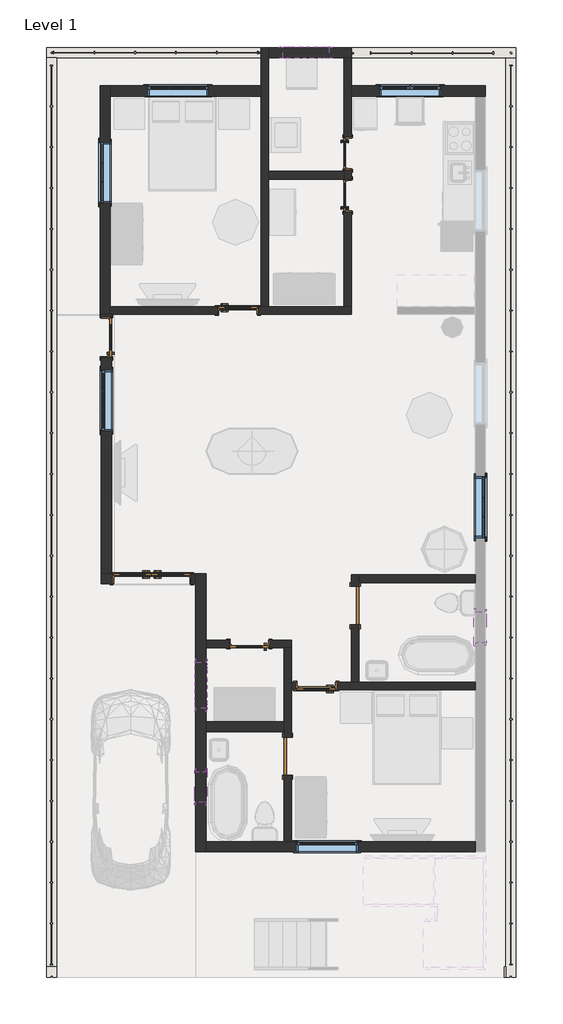
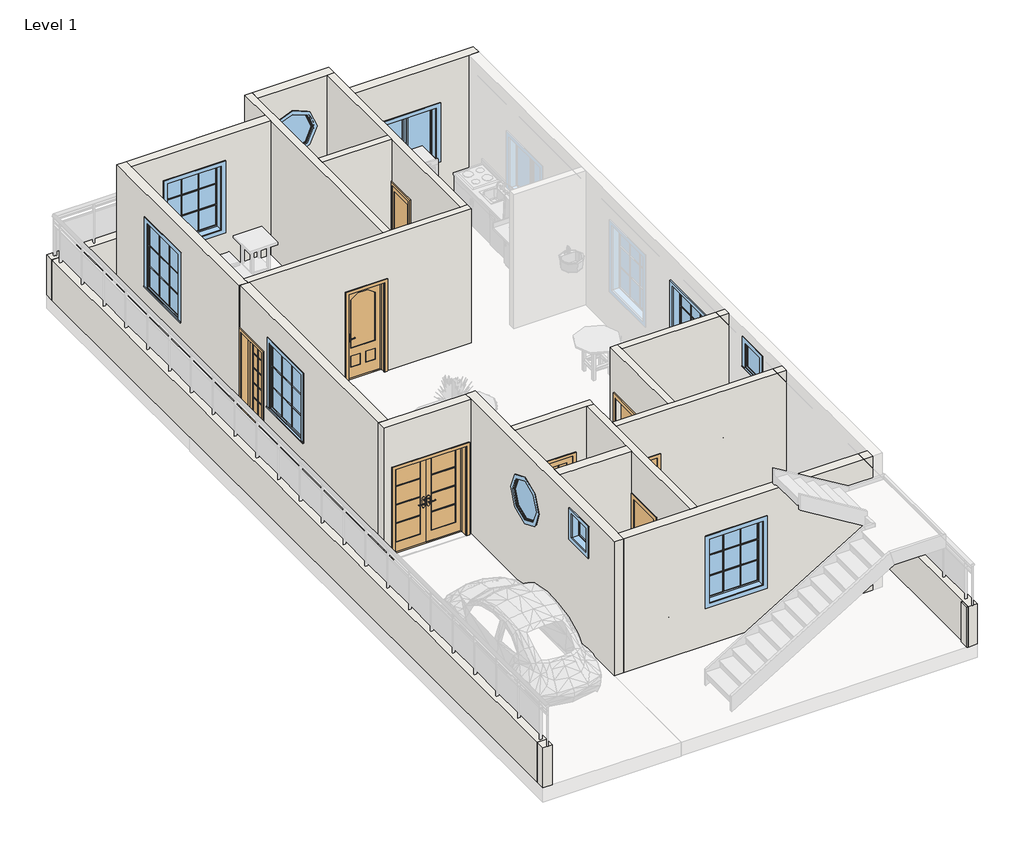
# One storey, part 1 of 3: 24 walls, 10 windows, 9 doors.
"""IFC4 building model written with IfcOpenShell, lengths in millimetres."""

from ifc_helpers import new_model, si_unit, frame, origin, origin_with_axes, place, context, project, spatial, polyline, circle_curve, outline, extrude, faceted_brep, transform, mapped, element, save
from ifc_brep_helpers import plane_surface, revolved_surface, advanced_brep
from components import door_4b146b56, door_b03bd389, door_6ed77e8d, door_1d623f84, door_d788789e, door_fa41f557, door_059fdd7e, door_255cab33, window_cfa1ffdd, window_0862ab64, window_736d8d37, window_e41d21a6

model = new_model("IFC4")

# Units and contexts
model_context = context("Model", 3, world=origin())
ifc_project = project(units=[si_unit("LENGTHUNIT", "METRE", prefix="MILLI")], contexts=[model_context])

# Site, building, storey
site = spatial("IfcSite", under=ifc_project)
building = spatial("IfcBuilding", under=site)
storey = spatial("IfcBuildingStorey", under=building, Name="Level 1", Elevation=0.0)

# Doors
placement = place(None, origin())
door_shape = door_4b146b56(model_context)
element("IfcDoor", 1, ObjectType="30\" x 80\"", at=placement, inside=storey, context=model_context, shape_type="MappedRepresentation", body=[
    mapped(door_shape, transform((-3967.408395, 10244.7901182, 0.0), x_axis=(-1.0, 0.0, 0.0), y_axis=(0.0, -1.0, 0.0), z_axis=(0.0, 0.0, 1.0))),
])
element("IfcDoor", 2, ObjectType="30\" x 80\"", at=placement, inside=storey, context=model_context, shape_type="MappedRepresentation", body=[
    mapped(door_shape, transform((-2405.308395, 2770.8401182, 0.0), x_axis=(1.0, 0.0, 0.0), y_axis=(0.0, 1.0, 0.0), z_axis=(0.0, 0.0, 1.0))),
])
door_2_shape = door_b03bd389(model_context)
element("IfcDoor", 3, ObjectType="Door-Exterior-Double-Full Glass-Wood_Clad : 60\" x 80\"", at=placement, inside=storey, context=model_context, shape_type="MappedRepresentation", body=[
    mapped(door_2_shape, transform((-5681.908395, 4910.7901182, 0.0), x_axis=(1.0, 0.0, 0.0), y_axis=(0.0, 1.0, 0.0), z_axis=(0.0, 0.0, 1.0))),
])
door_3_shape = door_6ed77e8d(model_context)
element("IfcDoor", 4, ObjectType="Door-Interior-Single-1_Panel-Wood : 24\" x 80\"", at=placement, inside=storey, context=model_context, shape_type="MappedRepresentation", body=[
    mapped(door_3_shape, transform((-1786.183395, 12527.6151182, 0.0), x_axis=(0.0, 1.0, 0.0), y_axis=(-1.0, 0.0, 0.0), z_axis=(0.0, 0.0, 1.0))),
])
door_4_shape = door_1d623f84(model_context)
element("IfcDoor", 5, ObjectType="Door-Interior-Single-1_Panel-Wood : 24\" x 80\"", at=placement, inside=storey, context=model_context, shape_type="MappedRepresentation", body=[
    mapped(door_4_shape, transform((-1786.183395, 13365.8151182, 0.0), x_axis=(0.0, -1.0, 0.0), y_axis=(1.0, 0.0, 0.0), z_axis=(0.0, 0.0, 1.0))),
])
door_5_shape = door_d788789e(model_context)
element("IfcDoor", 6, ObjectType="Door-Interior-Single-Full Glass-Wood : 30\" x 80\"", at=placement, inside=storey, context=model_context, shape_type="MappedRepresentation", body=[
    mapped(door_5_shape, transform((-6580.433395, 9708.2151182, 0.0), x_axis=(0.0, 1.0, 0.0), y_axis=(-1.0, 0.0, 0.0), z_axis=(0.0, 0.0, 1.0))),
])
door_6_shape = door_fa41f557(model_context)
element("IfcDoor", 7, ObjectType="Door-Interior-Single-Full Glass-Wood : 30\" x 80\"", at=placement, inside=storey, context=model_context, shape_type="MappedRepresentation", body=[
    mapped(door_6_shape, transform((-3738.808395, 3609.0401182, 0.0), x_axis=(-1.0, 0.0, 0.0), y_axis=(0.0, -1.0, 0.0), z_axis=(0.0, 0.0, 1.0))),
])
door_7_shape = door_059fdd7e(model_context)
element("IfcDoor", 8, ObjectType="Single-Flush : 30\" x 80\"", at=placement, inside=storey, context=model_context, shape_type="MappedRepresentation", body=[
    mapped(door_7_shape, transform((-2976.808395, 1377.0151182, 0.0), x_axis=(0.0, 1.0, 0.0), y_axis=(-1.0, 0.0, 0.0), z_axis=(0.0, 0.0, 1.0))),
])
door_8_shape = door_255cab33(model_context)
element("IfcDoor", 9, ObjectType="Single-Flush : 30\" x 80\"", at=placement, inside=storey, context=model_context, shape_type="MappedRepresentation", body=[
    mapped(door_8_shape, transform((-1630.608395, 4374.2151182, 0.0), x_axis=(0.0, 1.0, 0.0), y_axis=(-1.0, 0.0, 0.0), z_axis=(0.0, 0.0, 1.0))),
])

# Walls
element("IfcWall", 10, ObjectType="Generic - 8\"", at=placement, inside=storey, context=model_context, shape_type="SweptSolid", body=[
    extrude(outline(polyline([(1341.191605, -2813.9848818), (1366.591605, -2813.9848818), (1366.591605, -3017.1848818), (1341.191605, -3017.1848818), (1341.191605, -2813.9848818)])), origin_with_axes(), (0.0, 0.0, 1.0), 914.4),
])
element("IfcWall", 11, ObjectType="Generic - 8\"", at=placement, inside=storey, context=model_context, shape_type="Brep", body=[
    faceted_brep([(-6685.208395, 10165.4151182, 3048.0), (-6685.208395, 10165.4151182, 0.0), (-6685.208395, 10114.6151182, 0.0), (-6685.208395, 10114.6151182, 2057.4), (-6685.208395, 9301.8151182, 2057.4), (-6685.208395, 9301.8151182, 0.0), (-6685.208395, 5009.2151182, 0.0), (-6685.208395, 5009.2151182, 3048.0), (-6685.208395, 9060.5151182, 2438.4), (-6685.208395, 7841.3151182, 2438.4), (-6685.208395, 7841.3151182, 914.4), (-6685.208395, 9060.5151182, 914.4), (-6482.008395, 10165.4151182, 0.0), (-6482.008395, 10165.4151182, 3048.0), (-6482.008395, 5009.2151182, 3048.0), (-6482.008395, 5009.2151182, 0.0), (-6482.008395, 9301.8151182, 0.0), (-6482.008395, 9301.8151182, 2057.4), (-6482.008395, 10114.6151182, 2057.4), (-6482.008395, 10114.6151182, 0.0), (-6482.008395, 9060.5151182, 2438.4), (-6482.008395, 9060.5151182, 914.4), (-6482.008395, 7841.3151182, 914.4), (-6482.008395, 7841.3151182, 2438.4), (-6507.408395, 10165.4151182, 0.0), (-6507.408395, 10165.4151182, 3048.0)], [[[0, 1, 2, 3, 4, 5, 6, 7], [8, 9, 10, 11]], [[12, 13, 14, 15, 16, 17, 18, 19], [20, 21, 22, 23]], [[15, 6, 5, 16]], [[1, 24, 12, 19, 2]], [[1, 0, 25, 13, 12, 24]], [[7, 6, 15, 14]], [[18, 3, 2, 19]], [[3, 18, 17, 4]], [[4, 17, 16, 5]], [[21, 20, 8, 11]], [[22, 21, 11, 10]], [[23, 22, 10, 9]], [[20, 23, 9, 8]], [[0, 7, 14, 13, 25]]]),
])
element("IfcWall", 12, ObjectType="Generic - 8\"", at=placement, inside=storey, context=model_context, shape_type="Brep", body=[
    faceted_brep([(-4805.608395, 5009.2151182, 3048.0), (-4805.608395, 5009.2151182, 0.0), (-4894.508395, 5009.2151182, 0.0), (-4894.508395, 5009.2151182, 2057.4), (-6469.308395, 5009.2151182, 2057.4), (-6469.308395, 5009.2151182, 0.0), (-6482.008395, 5009.2151182, 0.0), (-6685.208395, 5009.2151182, 0.0), (-6685.208395, 5009.2151182, 3048.0), (-6482.008395, 5009.2151182, 3048.0), (-4805.608395, 4806.0151182, 0.0), (-4805.608395, 4806.0151182, 3048.0), (-6685.208395, 4806.0151182, 3048.0), (-6685.208395, 4806.0151182, 0.0), (-6469.308395, 4806.0151182, 0.0), (-6469.308395, 4806.0151182, 2057.4), (-4894.508395, 4806.0151182, 2057.4), (-4894.508395, 4806.0151182, 0.0)], [[[0, 1, 2, 3, 4, 5, 6, 7, 8, 9]], [[10, 11, 12, 13, 14, 15, 16, 17]], [[1, 10, 17, 2]], [[13, 7, 6, 5, 14]], [[1, 0, 11, 10]], [[8, 7, 13, 12]], [[16, 3, 2, 17]], [[3, 16, 15, 4]], [[4, 15, 14, 5]], [[0, 9, 8, 12, 11]]]),
])
element("IfcWall", 13, ObjectType="Generic - 8\"", at=placement, inside=storey, context=model_context, shape_type="SweptSolid", body=[
    extrude(outline(polyline([(0.0, -6507.408395), (0.0, -3510.208395), (3048.0, -3510.208395), (3048.0, -6507.408395), (0.0, -6507.408395)]), holes=[polyline([(2438.4, -4551.608395), (914.4, -4551.608395), (914.4, -5770.808395), (2438.4, -5770.808395), (2438.4, -4551.608395)])]), frame((0.0, 14508.8151182, 0.0), z_axis=(0.0, 1.0, 0.0), x_axis=(0.0, 0.0, 1.0)), (0.0, 0.0, 1.0), 203.2),
])
element("IfcWall", 14, ObjectType="Generic - 8\"", at=placement, inside=storey, context=model_context, shape_type="Brep", body=[
    faceted_brep([(-1706.808395, 14508.8151182, 0.0), (756.991605, 14508.8151182, 0.0), (960.191605, 14508.8151182, 0.0), (960.191605, 14508.8151182, 3048.0), (756.991605, 14508.8151182, 3048.0), (-1706.808395, 14508.8151182, 3048.0), (71.191605, 14508.8151182, 2133.6), (71.191605, 14508.8151182, 914.4), (-1148.008395, 14508.8151182, 914.4), (-1148.008395, 14508.8151182, 2133.6), (-1706.808395, 14712.0151182, 0.0), (-1706.808395, 14712.0151182, 3048.0), (960.191605, 14712.0151182, 3048.0), (960.191605, 14712.0151182, 0.0), (71.191605, 14712.0151182, 2133.6), (-1148.008395, 14712.0151182, 2133.6), (-1148.008395, 14712.0151182, 914.4), (71.191605, 14712.0151182, 914.4)], [[[0, 1, 2, 3, 4, 5], [6, 7, 8, 9]], [[10, 11, 12, 13], [14, 15, 16, 17]], [[2, 1, 0, 10, 13]], [[0, 5, 11, 10]], [[3, 2, 13, 12]], [[7, 6, 14, 17]], [[8, 7, 17, 16]], [[9, 8, 16, 15]], [[6, 9, 15, 14]], [[5, 4, 3, 12, 11]]]),
])
element("IfcWall", 15, ObjectType="Generic - 8\"", at=placement, inside=storey, context=model_context, shape_type="Brep", body=[
    faceted_brep([(756.991605, -324.7848818, 0.0), (-2900.608395, -324.7848818, 0.0), (-3053.008395, -324.7848818, 0.0), (-4602.408395, -324.7848818, 0.0), (-4602.408395, -324.7848818, 3048.0), (-3053.008395, -324.7848818, 3048.0), (-2900.608395, -324.7848818, 3048.0), (756.991605, -324.7848818, 3048.0), (-1579.808395, -324.7848818, 2438.4), (-2799.008395, -324.7848818, 2438.4), (-2799.008395, -324.7848818, 914.4), (-1579.808395, -324.7848818, 914.4), (756.991605, -527.9848818, 0.0), (756.991605, -527.9848818, 3048.0), (-4602.408395, -527.9848818, 3048.0), (-4602.408395, -527.9848818, 0.0), (-1579.808395, -527.9848818, 2438.4), (-1579.808395, -527.9848818, 914.4), (-2799.008395, -527.9848818, 914.4), (-2799.008395, -527.9848818, 2438.4)], [[[0, 1, 2, 3, 4, 5, 6, 7], [8, 9, 10, 11]], [[12, 13, 14, 15], [16, 17, 18, 19]], [[3, 2, 1, 0, 12, 15]], [[0, 7, 13, 12]], [[4, 3, 15, 14]], [[17, 16, 8, 11]], [[18, 17, 11, 10]], [[19, 18, 10, 9]], [[16, 19, 9, 8]], [[7, 6, 5, 4, 14, 13]]]),
])
element("IfcWall", 16, ObjectType="Generic - 8\"", at=placement, inside=storey, context=model_context, shape_type="Brep", body=[
    faceted_brep([(-6710.608395, 14712.0151182, 0.0), (-6710.608395, 10165.4151182, 0.0), (-6710.608395, 10165.4151182, 3048.0), (-6710.608395, 14712.0151182, 3048.0), (-6710.608395, 13594.4151182, 2438.4), (-6710.608395, 12375.2151182, 2438.4), (-6710.608395, 12375.2151182, 914.4), (-6710.608395, 13594.4151182, 914.4), (-6507.408395, 14712.0151182, 0.0), (-6507.408395, 14712.0151182, 3048.0), (-6507.408395, 14508.8151182, 3048.0), (-6507.408395, 10317.8151182, 3048.0), (-6507.408395, 10165.4151182, 3048.0), (-6507.408395, 10165.4151182, 0.0), (-6507.408395, 10317.8151182, 0.0), (-6507.408395, 14508.8151182, 0.0), (-6507.408395, 13594.4151182, 2438.4), (-6507.408395, 13594.4151182, 914.4), (-6507.408395, 12375.2151182, 914.4), (-6507.408395, 12375.2151182, 2438.4), (-6685.208395, 10165.4151182, 0.0), (-6685.208395, 10165.4151182, 3048.0)], [[[0, 1, 2, 3], [4, 5, 6, 7]], [[8, 9, 10, 11, 12, 13, 14, 15], [16, 17, 18, 19]], [[1, 0, 8, 15, 14, 13, 20]], [[2, 1, 20, 13, 12, 21]], [[0, 3, 9, 8]], [[17, 16, 4, 7]], [[18, 17, 7, 6]], [[19, 18, 6, 5]], [[16, 19, 5, 4]], [[3, 2, 21, 12, 11, 10, 9]]]),
])
element("IfcWall", 17, ObjectType="Generic - 8\"", at=placement, inside=storey, context=model_context, shape_type="AdvancedBrep", body=[
    advanced_brep(
    [(-4602.408395, -527.9848818, 0.0), (-4602.408395, -324.7848818, 0.0), (-4602.408395, 1859.6151182, 0.0), (-4602.408395, 2062.8151182, 0.0), (-4602.408395, 3536.0151182, 0.0), (-4602.408395, 3688.4151182, 0.0), (-4602.408395, 5009.2151182, 0.0), (-4602.408395, 5009.2151182, 3048.0), (-4602.408395, 3688.4151182, 3048.0), (-4602.408395, 3536.0151182, 3048.0), (-4602.408395, 2062.8151182, 3048.0), (-4602.408395, 1859.6151182, 3048.0), (-4602.408395, -324.7848818, 3048.0), (-4602.408395, -527.9848818, 3048.0), (-4602.408395, 462.6151182, 2768.6), (-4602.408395, 1072.2151182, 2768.6), (-4602.408395, 1072.2151182, 2159.0), (-4602.408395, 462.6151182, 2159.0), (-4602.408395, 2329.5151182, 1981.2), (-4602.408395, 3243.9151182, 1981.2), (-4805.608395, -527.9848818, 0.0), (-4805.608395, -527.9848818, 3048.0), (-4805.608395, 4806.0151182, 3048.0), (-4805.608395, 5009.2151182, 3048.0), (-4805.608395, 5009.2151182, 0.0), (-4805.608395, 4806.0151182, 0.0), (-4805.608395, 462.6151182, 2768.6), (-4805.608395, 462.6151182, 2159.0), (-4805.608395, 1072.2151182, 2159.0), (-4805.608395, 1072.2151182, 2768.6), (-4805.608395, 2329.5151182, 1981.2), (-4805.608395, 3243.9151182, 1981.2)],
    [
        (0, 1),
        (1, 2),
        (2, 3),
        (3, 4),
        (4, 5),
        (5, 6),
        (6, 7),
        (7, 8),
        (8, 9),
        (9, 10),
        (10, 11),
        (11, 12),
        (12, 13),
        (13, 0),
        (14, 15),
        (15, 16),
        (16, 17),
        (17, 14),
        (18, 19, circle_curve(frame((-4602.408395, 2786.7151182, 1981.2), z_axis=(-1.0, 0.0, 0.0), x_axis=(0.0, 1.0, 0.0)), 457.2)),
        (19, 18, circle_curve(frame((-4602.408395, 2786.7151182, 1981.2), z_axis=(-1.0, 0.0, 0.0), x_axis=(0.0, 1.0, 0.0)), 457.2)),
        (20, 21),
        (21, 22),
        (22, 23),
        (23, 24),
        (24, 25),
        (25, 20),
        (26, 27),
        (27, 28),
        (28, 29),
        (29, 26),
        (30, 31, circle_curve(frame((-4805.608395, 2786.7151182, 1981.2), z_axis=(1.0, 0.0, 0.0), x_axis=(0.0, 1.0, 0.0)), 457.2)),
        (31, 30, circle_curve(frame((-4805.608395, 2786.7151182, 1981.2), z_axis=(1.0, 0.0, 0.0), x_axis=(0.0, 1.0, 0.0)), 457.2)),
        (0, 20),
        (24, 6),
        (23, 7),
        (13, 21),
        (26, 14),
        (17, 27),
        (16, 28),
        (15, 29),
        (30, 18),
        (19, 31),
    ],
    [
        plane_surface(frame((-4602.408395, -2864.7848818, 0.0), z_axis=(1.0, 0.0, 0.0), x_axis=(0.0, 1.0, 0.0))),
        plane_surface(frame((-4805.608395, -2864.7848818, 0.0), z_axis=(-1.0, 0.0, 0.0), x_axis=(0.0, -1.0, 0.0))),
        plane_surface(frame((-4602.408395, -426.3848818, 0.0), z_axis=(0.0, 0.0, -1.0), x_axis=(-1.0, 0.0, 0.0))),
        plane_surface(frame((-4196.008395, 5009.2151182, 0.0), z_axis=(0.0, 1.0, 0.0), x_axis=(-1.0, 0.0, 0.0))),
        plane_surface(frame((858.591605, -527.9848818, 0.0), z_axis=(0.0, -1.0, 0.0), x_axis=(1.0, 0.0, 0.0))),
        plane_surface(frame((-7777.408395, 15474.0151182, 3048.0), z_axis=(0.0, 0.0, 1.0), x_axis=(1.0, 0.0, 0.0))),
        plane_surface(frame((-4805.608395, 462.6151182, 2768.6), z_axis=(0.0, 1.0, 0.0), x_axis=(1.0, 0.0, 0.0))),
        plane_surface(frame((-4805.608395, 462.6151182, 2159.0), z_axis=(0.0, 0.0, 1.0), x_axis=(1.0, 0.0, 0.0))),
        plane_surface(frame((-4805.608395, 1072.2151182, 2159.0), z_axis=(0.0, -1.0, 0.0), x_axis=(1.0, 0.0, 0.0))),
        plane_surface(frame((-4805.608395, 1072.2151182, 2768.6), z_axis=(0.0, 0.0, -1.0), x_axis=(1.0, 0.0, 0.0))),
        revolved_surface(polyline([(-4602.408395, 3243.9151181999996, 1981.2), (-4805.608395, 3243.9151181999996, 1981.2)]), (-4602.408395, 2786.7151182, 1981.2), (1.0, 0.0, 0.0)),
    ],
    [
        (0, [[1, 2, 3, 4, 5, 6, 7, 8, 9, 10, 11, 12, 13, 14], [15, 16, 17, 18], [19, 20]]),
        (1, [[21, 22, 23, 24, 25, 26], [27, 28, 29, 30], [31, 32]]),
        (2, [[-6, -5, -4, -3, -2, -1, 33, -26, -25, 34]]),
        (3, [[-7, -34, -24, 35]]),
        (4, [[-14, 36, -21, -33]]),
        (5, [[-13, -12, -11, -10, -9, -8, -35, -23, -22, -36]]),
        (6, [[-27, 37, -18, 38]]),
        (7, [[-28, -38, -17, 39]]),
        (8, [[-29, -39, -16, 40]]),
        (9, [[-30, -40, -15, -37]]),
        (10, [[-31, 41, -20, 42]]),
        (10, [[-32, -42, -19, -41]]),
    ],
),
])
element("IfcWall", 18, ObjectType="Generic - 8\"", at=placement, inside=storey, context=model_context, shape_type="SweptSolid", body=[
    extrude(outline(polyline([(-4602.408395, 2062.8151182), (-3053.008395, 2062.8151182), (-3053.008395, 1859.6151182), (-4602.408395, 1859.6151182), (-4602.408395, 2062.8151182)])), origin_with_axes(), (0.0, 0.0, 1.0), 3048.0),
])
element("IfcWall", 19, ObjectType="INNER WALL", at=placement, inside=storey, context=model_context, shape_type="Brep", body=[
    faceted_brep([(-1706.808395, 10165.4151182, 0.0), (-1706.808395, 10165.4151182, 3048.0), (-6482.008395, 10165.4151182, 3048.0), (-6507.408395, 10165.4151182, 3048.0), (-6507.408395, 10165.4151182, 0.0), (-6482.008395, 10165.4151182, 0.0), (-4373.808395, 10165.4151182, 0.0), (-4373.808395, 10165.4151182, 2057.4), (-3561.008395, 10165.4151182, 2057.4), (-3561.008395, 10165.4151182, 0.0), (-1706.808395, 10317.8151182, 3048.0), (-1706.808395, 10317.8151182, 0.0), (-1859.208395, 10317.8151182, 0.0), (-3357.808395, 10317.8151182, 0.0), (-3510.208395, 10317.8151182, 0.0), (-3561.008395, 10317.8151182, 0.0), (-3561.008395, 10317.8151182, 2057.4), (-4373.808395, 10317.8151182, 2057.4), (-4373.808395, 10317.8151182, 0.0), (-6507.408395, 10317.8151182, 0.0), (-6507.408395, 10317.8151182, 3048.0), (-3510.208395, 10317.8151182, 3048.0), (-3357.808395, 10317.8151182, 3048.0), (-1859.208395, 10317.8151182, 3048.0)], [[[0, 1, 2, 3, 4, 5, 6, 7, 8, 9]], [[10, 11, 12, 13, 14, 15, 16, 17, 18, 19, 20, 21, 22, 23]], [[11, 0, 9, 15, 14, 13, 12]], [[4, 19, 18, 6, 5]], [[1, 0, 11, 10]], [[4, 3, 20, 19]], [[17, 7, 6, 18]], [[7, 17, 16, 8]], [[8, 16, 15, 9]], [[3, 2, 1, 10, 23, 22, 21, 20]]]),
])
element("IfcWall", 20, ObjectType="INNER WALL", at=placement, inside=storey, context=model_context, shape_type="Brep", body=[
    faceted_brep([(-3510.208395, 15270.8151182, 0.0), (-3510.208395, 14712.0151182, 0.0), (-3510.208395, 14508.8151182, 0.0), (-3510.208395, 10317.8151182, 0.0), (-3510.208395, 10317.8151182, 3048.0), (-3510.208395, 14508.8151182, 3048.0), (-3510.208395, 14712.0151182, 3048.0), (-3510.208395, 15474.0151182, 3048.0), (-3510.208395, 15474.0151182, 914.4), (-3510.208395, 15270.8151182, 914.4), (-3357.808395, 15270.8151182, 0.0), (-3357.808395, 15270.8151182, 914.4), (-3357.808395, 15474.0151182, 914.4), (-3357.808395, 15474.0151182, 3048.0), (-3357.808395, 15270.8151182, 3048.0), (-3357.808395, 13010.2151182, 3048.0), (-3357.808395, 12857.8151182, 3048.0), (-3357.808395, 10317.8151182, 3048.0), (-3357.808395, 10317.8151182, 0.0), (-3357.808395, 12857.8151182, 0.0), (-3357.808395, 13010.2151182, 0.0)], [[[0, 1, 2, 3, 4, 5, 6, 7, 8, 9]], [[10, 11, 12, 13, 14, 15, 16, 17, 18, 19, 20]], [[3, 2, 1, 0, 10, 20, 19, 18]], [[4, 3, 18, 17]], [[8, 12, 11, 9]], [[0, 9, 11, 10]], [[8, 7, 13, 12]], [[7, 6, 5, 4, 17, 16, 15, 14, 13]]]),
])
element("IfcWall", 21, ObjectType="INNER WALL", at=placement, inside=storey, context=model_context, shape_type="Brep", body=[
    faceted_brep([(-1859.208395, 10317.8151182, 0.0), (-1859.208395, 10317.8151182, 3048.0), (-1859.208395, 12857.8151182, 3048.0), (-1859.208395, 13010.2151182, 3048.0), (-1859.208395, 15270.8151182, 3048.0), (-1859.208395, 15270.8151182, 0.0), (-1859.208395, 13696.0151182, 0.0), (-1859.208395, 13696.0151182, 2057.4), (-1859.208395, 13035.6151182, 2057.4), (-1859.208395, 13035.6151182, 0.0), (-1859.208395, 13010.2151182, 0.0), (-1859.208395, 12857.8151182, 0.0), (-1859.208395, 12857.8151182, 2057.4), (-1859.208395, 12197.4151182, 2057.4), (-1859.208395, 12197.4151182, 0.0), (-1706.808395, 10317.8151182, 3048.0), (-1706.808395, 10317.8151182, 0.0), (-1706.808395, 12197.4151182, 0.0), (-1706.808395, 12197.4151182, 2057.4), (-1706.808395, 12857.8151182, 2057.4), (-1706.808395, 12857.8151182, 0.0), (-1706.808395, 13035.6151182, 0.0), (-1706.808395, 13035.6151182, 2057.4), (-1706.808395, 13696.0151182, 2057.4), (-1706.808395, 13696.0151182, 0.0), (-1706.808395, 14508.8151182, 0.0), (-1706.808395, 14712.0151182, 0.0), (-1706.808395, 15270.8151182, 0.0), (-1706.808395, 15270.8151182, 914.4), (-1706.808395, 15270.8151182, 3048.0), (-1706.808395, 14712.0151182, 3048.0), (-1706.808395, 14508.8151182, 3048.0), (-1783.008395, 15270.8151182, 0.0)], [[[0, 1, 2, 3, 4, 5, 6, 7, 8, 9, 10, 11, 12, 13, 14]], [[15, 16, 17, 18, 19, 20, 21, 22, 23, 24, 25, 26, 27, 28, 29, 30, 31]], [[16, 0, 14, 17]], [[5, 32, 27, 26, 25, 24, 6]], [[20, 11, 10, 9, 21]], [[1, 0, 16, 15]], [[27, 32, 5, 4, 29, 28]], [[19, 12, 11, 20]], [[12, 19, 18, 13]], [[13, 18, 17, 14]], [[8, 22, 21, 9]], [[22, 8, 7, 23]], [[23, 7, 6, 24]], [[4, 3, 2, 1, 15, 31, 30, 29]]]),
])
element("IfcWall", 22, ObjectType="INNER WALL", at=placement, inside=storey, context=model_context, shape_type="Brep", body=[
    faceted_brep([(-1859.208395, 13010.2151182, 0.0), (-3357.808395, 13010.2151182, 0.0), (-3357.808395, 13010.2151182, 3048.0), (-1859.208395, 13010.2151182, 3048.0), (-1859.208395, 12857.8151182, 0.0), (-1859.208395, 12857.8151182, 2057.4), (-1859.208395, 12857.8151182, 3048.0), (-3357.808395, 12857.8151182, 3048.0), (-3357.808395, 12857.8151182, 0.0)], [[[0, 1, 2, 3]], [[4, 5, 6, 7, 8]], [[1, 0, 4, 8]], [[0, 3, 6, 5, 4]], [[2, 1, 8, 7]], [[3, 2, 7, 6]]]),
])
element("IfcWall", 23, ObjectType="INNER WALL", at=placement, inside=storey, context=model_context, shape_type="Brep", body=[
    faceted_brep([(-4602.408395, 3536.0151182, 3048.0), (-4602.408395, 3536.0151182, 0.0), (-4145.208395, 3536.0151182, 0.0), (-4145.208395, 3536.0151182, 2057.4), (-3332.408395, 3536.0151182, 2057.4), (-3332.408395, 3536.0151182, 0.0), (-3053.008395, 3536.0151182, 0.0), (-2900.608395, 3536.0151182, 0.0), (-2900.608395, 3536.0151182, 3048.0), (-3053.008395, 3536.0151182, 3048.0), (-4602.408395, 3688.4151182, 0.0), (-4602.408395, 3688.4151182, 3048.0), (-2900.608395, 3688.4151182, 3048.0), (-2900.608395, 3688.4151182, 0.0), (-3332.408395, 3688.4151182, 0.0), (-3332.408395, 3688.4151182, 2057.4), (-4145.208395, 3688.4151182, 2057.4), (-4145.208395, 3688.4151182, 0.0)], [[[0, 1, 2, 3, 4, 5, 6, 7, 8, 9]], [[10, 11, 12, 13, 14, 15, 16, 17]], [[1, 10, 17, 2]], [[13, 7, 6, 5, 14]], [[1, 0, 11, 10]], [[8, 7, 13, 12]], [[16, 3, 2, 17]], [[3, 16, 15, 4]], [[4, 15, 14, 5]], [[0, 9, 8, 12, 11]]]),
])
element("IfcWall", 24, ObjectType="INNER WALL", at=placement, inside=storey, context=model_context, shape_type="Brep", body=[
    faceted_brep([(-3053.008395, 3536.0151182, 0.0), (-3053.008395, 2062.8151182, 0.0), (-3053.008395, 1859.6151182, 0.0), (-3053.008395, 1758.0151182, 0.0), (-3053.008395, 1758.0151182, 2032.0), (-3053.008395, 996.0151182, 2032.0), (-3053.008395, 996.0151182, 0.0), (-3053.008395, -324.7848818, 0.0), (-3053.008395, -324.7848818, 3048.0), (-3053.008395, 1859.6151182, 3048.0), (-3053.008395, 2062.8151182, 3048.0), (-3053.008395, 3536.0151182, 3048.0), (-2900.608395, 1758.0151182, 2032.0), (-2900.608395, 1758.0151182, 0.0), (-2900.608395, 2697.8151182, 0.0), (-2900.608395, 2850.2151182, 0.0), (-2900.608395, 3536.0151182, 0.0), (-2900.608395, 3536.0151182, 3048.0), (-2900.608395, 2850.2151182, 3048.0), (-2900.608395, 2697.8151182, 3048.0), (-2900.608395, -324.7848818, 3048.0), (-2900.608395, -324.7848818, 0.0), (-2900.608395, 996.0151182, 0.0), (-2900.608395, 996.0151182, 2032.0)], [[[0, 1, 2, 3, 4, 5, 6, 7, 8, 9, 10, 11]], [[12, 13, 14, 15, 16, 17, 18, 19, 20, 21, 22, 23]], [[22, 21, 7, 6]], [[16, 15, 14, 13, 3, 2, 1, 0]], [[0, 11, 17, 16]], [[8, 7, 21, 20]], [[4, 3, 13, 12]], [[5, 4, 12, 23]], [[6, 5, 23, 22]], [[11, 10, 9, 8, 20, 19, 18, 17]]]),
])
element("IfcWall", 25, ObjectType="INNER WALL", at=placement, inside=storey, context=model_context, shape_type="Brep", body=[
    faceted_brep([(756.991605, 2697.8151182, 0.0), (756.991605, 2697.8151182, 3048.0), (-2900.608395, 2697.8151182, 3048.0), (-2900.608395, 2697.8151182, 0.0), (-2811.708395, 2697.8151182, 0.0), (-2811.708395, 2697.8151182, 2057.4), (-1998.908395, 2697.8151182, 2057.4), (-1998.908395, 2697.8151182, 0.0), (756.991605, 2850.2151182, 3048.0), (756.991605, 2850.2151182, 0.0), (-1554.408395, 2850.2151182, 0.0), (-1706.808395, 2850.2151182, 0.0), (-1998.908395, 2850.2151182, 0.0), (-1998.908395, 2850.2151182, 2057.4), (-2811.708395, 2850.2151182, 2057.4), (-2811.708395, 2850.2151182, 0.0), (-2900.608395, 2850.2151182, 0.0), (-2900.608395, 2850.2151182, 3048.0), (-1706.808395, 2850.2151182, 3048.0), (-1554.408395, 2850.2151182, 3048.0)], [[[0, 1, 2, 3, 4, 5, 6, 7]], [[8, 9, 10, 11, 12, 13, 14, 15, 16, 17, 18, 19]], [[3, 16, 15, 4]], [[9, 0, 7, 12, 11, 10]], [[1, 0, 9, 8]], [[3, 2, 17, 16]], [[6, 13, 12, 7]], [[13, 6, 5, 14]], [[14, 5, 4, 15]], [[2, 1, 8, 19, 18, 17]]]),
])
element("IfcWall", 26, ObjectType="INNER WALL", at=placement, inside=storey, context=model_context, shape_type="Brep", body=[
    faceted_brep([(-1554.408395, 4755.2151182, 2032.0), (-1554.408395, 4755.2151182, 0.0), (-1554.408395, 4831.4151182, 0.0), (-1554.408395, 4983.8151182, 0.0), (-1554.408395, 4983.8151182, 3048.0), (-1554.408395, 4831.4151182, 3048.0), (-1554.408395, 2850.2151182, 3048.0), (-1554.408395, 2850.2151182, 0.0), (-1554.408395, 3993.2151182, 0.0), (-1554.408395, 3993.2151182, 2032.0), (-1706.808395, 4983.8151182, 0.0), (-1706.808395, 4755.2151182, 0.0), (-1706.808395, 4755.2151182, 2032.0), (-1706.808395, 3993.2151182, 2032.0), (-1706.808395, 3993.2151182, 0.0), (-1706.808395, 2850.2151182, 0.0), (-1706.808395, 2850.2151182, 3048.0), (-1706.808395, 4983.8151182, 3048.0)], [[[0, 1, 2, 3, 4, 5, 6, 7, 8, 9]], [[10, 11, 12, 13, 14, 15, 16, 17]], [[8, 7, 15, 14]], [[3, 2, 1, 11, 10]], [[7, 6, 16, 15]], [[4, 3, 10, 17]], [[12, 11, 1, 0]], [[13, 12, 0, 9]], [[14, 13, 9, 8]], [[6, 5, 4, 17, 16]]]),
])
element("IfcWall", 27, ObjectType="INNER WALL", at=placement, inside=storey, context=model_context, shape_type="SweptSolid", body=[
    extrude(outline(polyline([(756.991605, 4831.4151182), (-1554.408395, 4831.4151182), (-1554.408395, 4983.8151182), (756.991605, 4983.8151182), (756.991605, 4831.4151182)])), origin_with_axes(), (0.0, 0.0, 1.0), 3048.0),
])
element("IfcWall", 28, ObjectType="OUTER WALL", at=placement, inside=storey, context=model_context, shape_type="Brep", body=[
    faceted_brep([(-7777.408395, 15270.8151182, 0.0), (-7574.208395, 15270.8151182, 0.0), (-3510.208395, 15270.8151182, 0.0), (-3357.808395, 15270.8151182, 0.0), (-3307.008395, 15270.8151182, 0.0), (-3307.008395, 15270.8151182, 914.4), (-3357.808395, 15270.8151182, 914.4), (-3510.208395, 15270.8151182, 914.4), (-7574.208395, 15270.8151182, 914.4), (-7777.408395, 15270.8151182, 914.4), (-7777.408395, 15474.0151182, 0.0), (-7777.408395, 15474.0151182, 914.4), (-3307.008395, 15474.0151182, 914.4), (-3307.008395, 15474.0151182, 0.0)], [[[0, 1, 2, 3, 4, 5, 6, 7, 8, 9]], [[10, 11, 12, 13]], [[4, 3, 2, 1, 0, 10, 13]], [[5, 4, 13, 12]], [[9, 8, 7, 6, 5, 12, 11]], [[0, 9, 11, 10]]]),
])
element("IfcWall", 29, ObjectType="OUTER WALL", at=placement, inside=storey, context=model_context, shape_type="Brep", body=[
    faceted_brep([(1366.591605, 15270.8151182, 0.0), (1366.591605, -2813.9848818, 0.0), (1366.591605, -3017.1848818, 0.0), (1366.591605, -3017.1848818, 914.4), (1366.591605, -2813.9848818, 914.4), (1366.591605, 15270.8151182, 914.4), (1569.791605, 15270.8151182, 0.0), (1569.791605, 15270.8151182, 914.4), (1569.791605, -3017.1848818, 914.4), (1569.791605, -3017.1848818, 0.0)], [[[0, 1, 2, 3, 4, 5]], [[6, 7, 8, 9]], [[2, 1, 0, 6, 9]], [[5, 4, 3, 8, 7]], [[0, 5, 7, 6]], [[3, 2, 9, 8]]]),
])
element("IfcWall", 30, ObjectType="OUTER WALL", at=placement, inside=storey, context=model_context, shape_type="SweptSolid", body=[
    extrude(outline(polyline([(-7574.208395, 15270.8151182), (-7574.208395, -2813.9848818), (-7777.408395, -2813.9848818), (-7777.408395, 15270.8151182), (-7574.208395, 15270.8151182)])), origin_with_axes(), (0.0, 0.0, 1.0), 914.4),
])
element("IfcWall", 31, ObjectType="OUTER WALL", at=placement, inside=storey, context=model_context, shape_type="SweptSolid", body=[
    extrude(outline(polyline([(-7777.408395, -2813.9848818), (-7574.208395, -2813.9848818), (-7574.208395, -3017.1848818), (-7777.408395, -3017.1848818), (-7777.408395, -2813.9848818)])), origin_with_axes(), (0.0, 0.0, 1.0), 914.4),
])
element("IfcWall", 32, ObjectType="OUTER WALL", at=placement, inside=storey, context=model_context, shape_type="Brep", body=[
    faceted_brep([(-1783.008395, 15270.8151182, 0.0), (-1706.808395, 15270.8151182, 0.0), (1366.591605, 15270.8151182, 0.0), (1569.791605, 15270.8151182, 0.0), (1569.791605, 15270.8151182, 914.4), (1366.591605, 15270.8151182, 914.4), (-1706.808395, 15270.8151182, 914.4), (-1783.008395, 15270.8151182, 914.4), (-1783.008395, 15474.0151182, 0.0), (-1783.008395, 15474.0151182, 914.4), (-1706.808395, 15474.0151182, 914.4), (1569.791605, 15474.0151182, 914.4), (1569.791605, 15474.0151182, 0.0)], [[[0, 1, 2, 3, 4, 5, 6, 7]], [[8, 9, 10, 11, 12]], [[3, 2, 1, 0, 8, 12]], [[7, 6, 5, 4, 11, 10, 9]], [[0, 7, 9, 8]], [[4, 3, 12, 11]]]),
])
element("IfcWall", 33, ObjectType="OUTER WALL", at=placement, inside=storey, context=model_context, shape_type="AdvancedBrep", body=[
    advanced_brep(
    [(-3357.808395, 15270.8151182, 0.0), (-1859.208395, 15270.8151182, 0.0), (-1783.008395, 15270.8151182, 0.0), (-1783.008395, 15270.8151182, 914.4), (-1706.808395, 15270.8151182, 914.4), (-1706.808395, 15270.8151182, 3048.0), (-1859.208395, 15270.8151182, 3048.0), (-3357.808395, 15270.8151182, 3048.0), (-2151.308395, 15270.8151182, 1981.2), (-3065.708395, 15270.8151182, 1981.2), (-3357.808395, 15474.0151182, 0.0), (-3357.808395, 15474.0151182, 914.4), (-3357.808395, 15474.0151182, 3048.0), (-1706.808395, 15474.0151182, 3048.0), (-1706.808395, 15474.0151182, 914.4), (-1783.008395, 15474.0151182, 914.4), (-1783.008395, 15474.0151182, 0.0), (-2151.308395, 15474.0151182, 1981.2), (-3065.708395, 15474.0151182, 1981.2)],
    [
        (0, 1),
        (1, 2),
        (2, 3),
        (3, 4),
        (4, 5),
        (5, 6),
        (6, 7),
        (7, 0),
        (8, 9, circle_curve(frame((-2608.508395, 15270.8151182, 1981.2), z_axis=(0.0, 1.0, 0.0), x_axis=(-1.0, 0.0, 0.0)), 457.2)),
        (9, 8, circle_curve(frame((-2608.508395, 15270.8151182, 1981.2), z_axis=(0.0, 1.0, 0.0), x_axis=(-1.0, 0.0, 0.0)), 457.2)),
        (10, 11),
        (11, 12),
        (12, 13),
        (13, 14),
        (14, 15),
        (15, 16),
        (16, 10),
        (17, 18, circle_curve(frame((-2608.508395, 15474.0151182, 1981.2), z_axis=(0.0, -1.0, 0.0), x_axis=(-1.0, 0.0, 0.0)), 457.2)),
        (18, 17, circle_curve(frame((-2608.508395, 15474.0151182, 1981.2), z_axis=(0.0, -1.0, 0.0), x_axis=(-1.0, 0.0, 0.0)), 457.2)),
        (0, 10),
        (16, 2),
        (15, 3),
        (14, 4),
        (13, 5),
        (7, 12),
        (8, 17),
        (18, 9),
    ],
    [
        plane_surface(frame((-7650.408395, 15270.8151182, 0.0), z_axis=(0.0, -1.0, 0.0), x_axis=(1.0, 0.0, 0.0))),
        plane_surface(frame((-7650.408395, 15474.0151182, 0.0), z_axis=(0.0, 1.0, 0.0), x_axis=(-1.0, 0.0, 0.0))),
        plane_surface(frame((-3434.008395, 15270.8151182, 0.0), z_axis=(0.0, 0.0, -1.0), x_axis=(0.0, 1.0, 0.0))),
        plane_surface(frame((-1783.008395, 15270.8151182, 0.0), z_axis=(1.0, 0.0, 0.0), x_axis=(0.0, 1.0, 0.0))),
        plane_surface(frame((-1783.008395, 15270.8151182, 914.4), z_axis=(0.0, 0.0, -1.0), x_axis=(1.0, 0.0, 0.0))),
        plane_surface(frame((-1706.808395, 15372.4151182, 0.0), z_axis=(1.0, 0.0, 0.0), x_axis=(0.0, 1.0, 0.0))),
        plane_surface(frame((-3357.808395, 15372.4151182, 0.0), z_axis=(-1.0, 0.0, 0.0), x_axis=(0.0, 1.0, 0.0))),
        plane_surface(frame((-7777.408395, 15474.0151182, 3048.0), z_axis=(0.0, 0.0, 1.0), x_axis=(1.0, 0.0, 0.0))),
        revolved_surface(polyline([(-3065.7083949999997, 15474.0151182, 1981.2), (-3065.7083949999997, 15270.8151182, 1981.2)]), (-2608.508395, 15474.0151182, 1981.2), (0.0, 1.0, 0.0)),
    ],
    [
        (0, [[1, 2, 3, 4, 5, 6, 7, 8], [9, 10]]),
        (1, [[11, 12, 13, 14, 15, 16, 17], [18, 19]]),
        (2, [[-2, -1, 20, -17, 21]]),
        (3, [[-3, -21, -16, 22]]),
        (4, [[23, -4, -22, -15]]),
        (5, [[-5, -23, -14, 24]]),
        (6, [[-8, 25, -12, -11, -20]]),
        (7, [[-7, -6, -24, -13, -25]]),
        (8, [[-9, 26, -19, 27]]),
        (8, [[-10, -27, -18, -26]]),
    ],
),
])

# Windows
window_shape = window_cfa1ffdd(model_context)
element("IfcWindow", 34, ObjectType="Casement 3x3 with Trim : 48\" x 60\"", at=placement, inside=storey, context=model_context, shape_type="MappedRepresentation", body=[
    mapped(window_shape, transform((-2189.408395, -426.3848818, 304.8), x_axis=(1.0, 0.0, 0.0), y_axis=(0.0, 1.0, 0.0), z_axis=(0.0, 0.0, 1.0))),
])
element("IfcWindow", 35, ObjectType="Casement 3x3 with Trim : 48\" x 60\"", at=placement, inside=storey, context=model_context, shape_type="MappedRepresentation", body=[
    mapped(window_shape, transform((858.591605, 6330.0151182, 304.8), x_axis=(0.0, -1.0, 0.0), y_axis=(1.0, 0.0, 0.0), z_axis=(0.0, 0.0, 1.0))),
])
element("IfcWindow", 36, ObjectType="Casement 3x3 with Trim : 48\" x 60\"", at=placement, inside=storey, context=model_context, shape_type="MappedRepresentation", body=[
    mapped(window_shape, transform((-5161.208395, 14610.4151182, 304.8), x_axis=(1.0, 0.0, 0.0), y_axis=(0.0, 1.0, 0.0), z_axis=(0.0, 0.0, 1.0))),
])
element("IfcWindow", 37, ObjectType="Casement 3x3 with Trim : 48\" x 60\"", at=placement, inside=storey, context=model_context, shape_type="MappedRepresentation", body=[
    mapped(window_shape, transform((-6609.008395, 12984.8151182, 304.8), x_axis=(0.0, 1.0, 0.0), y_axis=(-1.0, 0.0, 0.0), z_axis=(0.0, 0.0, 1.0))),
])
element("IfcWindow", 38, ObjectType="Casement 3x3 with Trim : 48\" x 60\"", at=placement, inside=storey, context=model_context, shape_type="MappedRepresentation", body=[
    mapped(window_shape, transform((-6583.608395, 8450.9151182, 304.8), x_axis=(0.0, 1.0, 0.0), y_axis=(-1.0, 0.0, 0.0), z_axis=(0.0, 0.0, 1.0))),
])
window_2_shape = window_0862ab64(model_context)
element("IfcWindow", 39, ObjectType="Casement Dbl with Trim : 48\" x 48\"", at=placement, inside=storey, context=model_context, shape_type="MappedRepresentation", body=[
    mapped(window_2_shape, transform((-538.408395, 14591.3651182, 0.0), x_axis=(1.0, 0.0, 0.0), y_axis=(0.0, 1.0, 0.0), z_axis=(0.0, 0.0, 1.0))),
])
window_3_shape = window_736d8d37(model_context)
element("IfcWindow", 40, ObjectType="Round with Trim : 36\" Diameter", at=placement, inside=storey, context=model_context, shape_type="MappedRepresentation", body=[
    mapped(window_3_shape, transform((-4704.008395, 2786.7151182, 762.0), x_axis=(0.0, 1.0, 0.0), y_axis=(-1.0, 0.0, 0.0), z_axis=(0.0, 0.0, 1.0))),
])
element("IfcWindow", 41, ObjectType="Round with Trim : 36\" Diameter", at=placement, inside=storey, context=model_context, shape_type="MappedRepresentation", body=[
    mapped(window_3_shape, transform((-2608.508395, 15372.4151182, 762.0), x_axis=(-1.0, 0.0, 0.0), y_axis=(0.0, -1.0, 0.0), z_axis=(0.0, 0.0, 1.0))),
])
window_4_shape = window_e41d21a6(model_context)
element("IfcWindow", 42, ObjectType="Transom with Trim : 24\" x 24\"", at=placement, inside=storey, context=model_context, shape_type="MappedRepresentation", body=[
    mapped(window_4_shape, transform((858.591605, 3980.5151182, 0.0), x_axis=(0.0, 1.0, 0.0), y_axis=(-1.0, 0.0, 0.0), z_axis=(0.0, 0.0, 1.0))),
])
element("IfcWindow", 43, ObjectType="Transom with Trim : 24\" x 24\"", at=placement, inside=storey, context=model_context, shape_type="MappedRepresentation", body=[
    mapped(window_4_shape, transform((-4704.008395, 729.3151182, 0.0), x_axis=(0.0, -1.0, 0.0), y_axis=(1.0, 0.0, 0.0), z_axis=(0.0, 0.0, 1.0))),
])

save(model, "model.ifc")

# Revit data of these elements
# Type "30\" x 80\""
#   Type Mark = "9"
#   Assembly Code = "B2030100"
#   Analytic Construction = "French door, wood frame with single glass"
#   Threshold Offset [instance default] = 0' - 0 1/2"
#   Thickness = 0' - 1 3/8"
#   Thermal Resistance (R) = 1.0696 (h·ft²·°F)/BTU
#   Swing Angle [instance default] = 90.00°
#   Stiles = 0' - 4 3/4"
#   Rough Width = 2' - 8"
#   Rough Height = 6' - 9"
#   Radius = 1' - 1.00625"
#   Lock Rail = 0' - 7 1/8"
#   Height = 6' - 8"
#   Width = 2' - 6"
#   Heat Transfer Coefficient (U) = 0.9350 BTU/(h·ft²·°F)
#   Door Offset [instance default] = 0' - 0"
#   Bottom Rail = 0' - 9 1/2"
#   Threshold [instance default] = yes
#   Function = 1
#   Exterior Trim [instance default] = yes
#   Trim Material = Cherry
#   Threshold Material = Cherry
#   Panel Material = Cherry
#   Glazing = Glass
#   Frame Material = Cherry
#   Door Handle Material = Aluminum
#   Visual Light Transmittance = 0
#   Solar Heat Gain Coefficient = 0
#   Wall Closure = (empty or 0)
#   Construction Type = (empty or 0)
# Type "Door-Exterior-Double-Full Glass-Wood_Clad : 60\" x 80\""
#   Type Mark = "8"
#   Assembly Code = "B2030100"
#   Analytic Construction = "French door, wood frame with double glass"
#   Top Rail = 0' - 4 11/16"
#   Threshold Offset [instance default] = 0' - 0 1/2"
#   Thickness = 0' - 1 3/8"
#   Thermal Resistance (R) = 1.9158 (h·ft²·°F)/BTU
#   Swing Angle [instance default] = 90.00°
#   Stiles = 0' - 4 3/4"
#   Rough Width = 5' - 2"
#   Rough Height = 6' - 9"
#   Panel Width = 2' - 6"
#   Door Offset [instance default] = 0' - 0"
#   Height = 6' - 8"
#   Width = 5' - 0"
#   Heat Transfer Coefficient (U) = 0.5220 BTU/(h·ft²·°F)
#   Bottom Rail = 0' - 9 1/8"
#   Exterior Trim [instance default] = yes
#   Threshold [instance default] = yes
#   Show Grill [instance default] = yes
#   Function = 1
#   Trim Material = Cherry
#   Threshold Material = Cherry
#   Panel Material = Cherry
#   Glazing = Glass
#   Frame Material = Cherry
#   Door Handle Material = Aluminum
#   Visual Light Transmittance = 0
#   Solar Heat Gain Coefficient = 0
#   Wall Closure = (empty or 0)
#   Construction Type = (empty or 0)
# Type "Door-Interior-Single-1_Panel-Wood : 24\" x 80\""
#   Type Mark = "12"
#   Assembly Code = "C1020300"
#   Analytic Construction = "Wooden"
#   Top Rail = 0' - 4 11/16"
#   Thickness = 0' - 1 3/8"
#   Thermal Resistance (R) = 2.5876 (h·ft²·°F)/BTU
#   Swing Angle [instance default] = 90.00°
#   Stiles = 0' - 2 3/8"
#   Rough Width = 2' - 2"
#   Rough Height = 6' - 9"
#   Height = 6' - 8"
#   Width = 2' - 0"
#   Heat Transfer Coefficient (U) = 0.3865 BTU/(h·ft²·°F)
#   Bottom Rail = 0' - 9 1/8"
#   Trim Material = Cherry
#   Panel Material = Cherry
#   Frame Material = Cherry
#   Door Handle Material = Aluminum
#   Visual Light Transmittance = 0
#   Solar Heat Gain Coefficient = 0
#   Wall Closure = (empty or 0)
#   Function = (empty or 0)
# Type "Door-Interior-Single-Full Glass-Wood : 30\" x 80\""
#   Type Mark = "10"
#   Assembly Code = "C1020300"
#   Analytic Construction = "Wood frame with single clear glass"
#   Top Rail = 0' - 4 11/16"
#   Thickness = 0' - 1 3/8"
#   Thermal Resistance (R) = 1.0102 (h·ft²·°F)/BTU
#   Swing Angle [instance default] = 90.00°
#   Stiles = 0' - 4 3/4"
#   Rough Width = 2' - 8"
#   Rough Height = 6' - 9"
#   Height = 6' - 8"
#   Width = 2' - 6"
#   Heat Transfer Coefficient (U) = 0.9900 BTU/(h·ft²·°F)
#   Bottom Rail = 0' - 9 1/8"
#   Show Grill [instance default] = yes
#   Trim Material = Cherry
#   Panel Material = Cherry
#   Frame Material = Cherry
#   Door Handle Material = Aluminum
#   Visual Light Transmittance = 0
#   Solar Heat Gain Coefficient = 0
#   Wall Closure = (empty or 0)
#   Function = (empty or 0)
# Type "Single-Flush : 30\" x 80\""
#   Type Mark = "5"
#   Construction Type Id = "MDOOR"
#   Assembly Code = "C1020"
#   Analytic Construction = "Metal"
#   Thickness = 0' - 2"
#   Heat Transfer Coefficient (U) = 0.651978 BTU/(h·ft²·°F)
#   Height = 6' - 8"
#   Trim Projection Ext = 0' - 1"
#   Trim Projection Int = 0' - 1"
#   Trim Width = 0' - 3"
#   Width = 2' - 6"
#   Define Thermal Properties by = 1
#   Door Material = Door - Panel
#   Frame Material = Door - Frame
#   Visual Light Transmittance = 0
#   Solar Heat Gain Coefficient = 0
#   Function = (empty or 0)
#   Wall Closure = (empty or 0)
# Type "Generic - 8\""
#   Assembly Code = "B2010"
#   Layers, outside or top first: 0' - 8" "Brick, Common" (function 1)
# Type "INNER WALL"
#   Assembly Code = "B2010"
#   Layers, outside or top first: 0' - 6" "Brick, Common" (function 1)
# Type "OUTER WALL"
#   Assembly Code = "B2010"
#   Layers, outside or top first: 0' - 8" "Brick, Soldier Course" (function 1)
# Type "Casement 3x3 with Trim : 48\" x 60\""
#   Type Mark = "11"
#   Construction Type Id = "GSP4R"
#   Assembly Code = "B2020100"
#   Analytic Construction = "1/8 in Pilkington single glazing"
#   Visual Light Transmittance = 0.9
#   Solar Heat Gain Coefficient = 0.78
#   Heat Transfer Coefficient (U) = 0.6496 BTU/(h·ft²·°F)
#   Height = 5' - 0"
#   Default Sill Height = 2' - 0"
#   Trim Projection - Ext. = 0' - 0 1/2"
#   Trim Projection - Int. = 0' - 0 3/4"
#   Trim Width - Exterior = 0' - 3 1/2"
#   Trim Width - Interior = 0' - 3 1/2"
#   Width = 4' - 0"
#   Window Inset = 0' - 0 3/4"
#   Define Thermal Properties by = 1
#   Glass Pane Material = Glass
#   Sash Material = Sash
#   Trim Exterior Material = Trim
#   Trim Interior Material = Trim
#   Wall Closure = (empty or 0)
# Type "Casement Dbl with Trim : 48\" x 48\""
#   Type Mark = "13"
#   Construction Type Id = "GSP4R"
#   Assembly Code = "B2020100"
#   Analytic Construction = "1/8 in Pilkington single glazing"
#   Visual Light Transmittance = 0.9
#   Solar Heat Gain Coefficient = 0.78
#   Heat Transfer Coefficient (U) = 0.6496 BTU/(h·ft²·°F)
#   Height = 4' - 0"
#   Default Sill Height = 3' - 0"
#   Trim Projection - Ext. = 0' - 0 1/2"
#   Trim Projection - Int. = 0' - 0 3/4"
#   Trim Width - Exterior = 0' - 3 1/2"
#   Trim Width - Interior = 0' - 3 1/2"
#   Width = 4' - 0"
#   Window Inset = 0' - 0 3/4"
#   Define Thermal Properties by = 1
#   Glass Pane Material = Glass
#   Sash Material = Sash
#   Trim Exterior Material = Trim
#   Trim Interior Material = Trim
#   Wall Closure = (empty or 0)
# Type "Round with Trim : 36\" Diameter"
#   Type Mark = "27"
#   Construction Type Id = "GSP4R"
#   Assembly Code = "B2020100"
#   Analytic Construction = "1/8 in Pilkington single glazing"
#   Visual Light Transmittance = 0.9
#   Solar Heat Gain Coefficient = 0.78
#   Heat Transfer Coefficient (U) = 0.6496 BTU/(h·ft²·°F)
#   Default Sill Height = 2' - 6"
#   Trim Projection - Ext. = 0' - 0 1/2"
#   Trim Projection - Int. = 0' - 0 3/4"
#   Trim Width - Exterior = 0' - 3 1/2"
#   Trim Width - Interior = 0' - 3 1/2"
#   Width = 3' - 0"
#   Define Thermal Properties by = 1
#   Glass Pane Material = Glass
#   Sash Material = Sash
#   Trim Exterior Material = Trim
#   Trim Interior Material = Trim
#   Wall Closure = (empty or 0)
# Type "Transom with Trim : 24\" x 24\""
#   Type Mark = "16"
#   Construction Type Id = "GSP4R"
#   Assembly Code = "B2020100"
#   Analytic Construction = "1/8 in Pilkington single glazing"
#   Visual Light Transmittance = 0.9
#   Solar Heat Gain Coefficient = 0.78
#   Heat Transfer Coefficient (U) = 0.6496 BTU/(h·ft²·°F)
#   Height = 2' - 0"
#   Default Sill Height = 7' - 1"
#   Trim Projection - Ext. = 0' - 0 1/2"
#   Trim Projection - Int. = 0' - 0 3/4"
#   Trim Width - Exterior = 0' - 3 1/2"
#   Trim Width - Interior = 0' - 3 1/2"
#   Width = 2' - 0"
#   Window Inset = 0' - 0 3/4"
#   Define Thermal Properties by = 1
#   Glass Pane Material = Glass
#   Sash Material = Sash
#   Trim Exterior Material = Trim
#   Trim Interior Material = Trim
#   Wall Closure = (empty or 0)
# Elements 1, 2 (IfcDoor, "30\" x 80\"")
#   Threshold Offset = 0' - 0 1/2"
#   Swing Angle = 90.00°
#   Door Offset = 0' - 0"
#   Threshold = yes
#   Exterior Trim = yes
#   Phase Created = New Construction
#   Materials on its faces: "Cherry", "Aluminum", "Glass"
# Element 3 (IfcDoor, "Door-Exterior-Double-Full Glass-Wood_Clad : 60\" x 80\"")
#   Threshold Offset = 0' - 0 1/2"
#   Swing Angle = 90.00°
#   Door Offset = 0' - 0"
#   Threshold = yes
#   Show Grill = yes
#   Exterior Trim = yes
#   Phase Created = New Construction
#   Materials on its faces: "Cherry", "Aluminum", "Glass"
# Elements 4, 5 (IfcDoor, "Door-Interior-Single-1_Panel-Wood : 24\" x 80\"")
#   Swing Angle = 90.00°
#   Phase Created = New Construction
#   Materials on its faces: "Cherry", "Aluminum"
# Elements 6, 7 (IfcDoor, "Door-Interior-Single-Full Glass-Wood : 30\" x 80\"")
#   Swing Angle = 90.00°
#   Show Grill = yes
#   Phase Created = New Construction
#   Materials on its faces: "Cherry", "Aluminum", "Glass"
# Elements 8, 9 (IfcDoor, "Single-Flush : 30\" x 80\"")
#   Phase Created = New Construction
#   Materials on its faces: "Door - Frame", "Door - Panel"
# Element 10 (IfcWall, "Generic - 8\"")
#   Top Offset = 0' - 0"
#   Base Offset = 0' - 0"
#   Unconnected Height = 3' - 0"
#   wall height = 3' - 0"
#   Phase Created = New Construction
#   Base Constraint = Level 1
#   Materials on its faces: "Brick, Common"
# Elements 11, 12, 13, 14, 15, 16, 17, 18 (IfcWall, "Generic - 8\"")
#   Top Offset = 0' - 0"
#   Base Offset = 0' - 0"
#   Unconnected Height = 10' - 0"
#   wall height = 10' - 0"
#   Phase Created = New Construction
#   Base Constraint = Level 1
#   Materials on its faces: "Brick, Common"
# Elements 19, 21, 22, 23, 24, 25, 26, 27 (IfcWall, "INNER WALL")
#   Top Offset = 0' - 0"
#   Base Offset = 0' - 0"
#   Unconnected Height = 10' - 0"
#   wall height = 10' - 0"
#   Phase Created = New Construction
#   Base Constraint = Level 1
#   Materials on its faces: "Brick, Common"
# Element 20 (IfcWall, "INNER WALL")
#   Top Offset = 0' - 0"
#   Base Offset = 0' - 0"
#   Unconnected Height = 10' - 0"
#   wall height = 10' - 0"
#   Phase Created = New Construction
#   Base Constraint = Level 1
#   Materials on its faces: "Brick, Common", "Brick, Soldier Course"
# Elements 28, 30, 31, 32 (IfcWall, "OUTER WALL")
#   Top Offset = 0' - 0"
#   Base Offset = 0' - 0"
#   Unconnected Height = 3' - 0"
#   wall height = 3' - 0"
#   Phase Created = New Construction
#   Base Constraint = Level 1
#   Materials on its faces: "Brick, Soldier Course"
# Element 29 (IfcWall, "OUTER WALL")
#   Top Offset = 0' - 0"
#   Base Offset = 0' - 0"
#   Unconnected Height = 3' - 0"
#   wall height = 3' - 0"
#   Phase Created = New Construction
#   Base Constraint = Level 1
#   Materials on its faces: "Brick, Soldier Course", "Brick, Common"
# Element 33 (IfcWall, "OUTER WALL")
#   Top Offset = 0' - 0"
#   Base Offset = 0' - 0"
#   Unconnected Height = 10' - 0"
#   wall height = 10' - 0"
#   Phase Created = New Construction
#   Base Constraint = Level 1
#   Materials on its faces: "Brick, Soldier Course", "Brick, Common"
# Element 34 (IfcWindow, "Casement 3x3 with Trim : 48\" x 60\"")
#   Mark = "1"
#   Phase Created = New Construction
#   Materials on its faces: "Sash", "Glass", "Trim"
# Element 35 (IfcWindow, "Casement 3x3 with Trim : 48\" x 60\"")
#   Mark = "2"
#   Phase Created = New Construction
#   Materials on its faces: "Sash", "Glass", "Trim"
# Element 36 (IfcWindow, "Casement 3x3 with Trim : 48\" x 60\"")
#   Mark = "4"
#   Phase Created = New Construction
#   Materials on its faces: "Sash", "Glass", "Trim"
# Element 37 (IfcWindow, "Casement 3x3 with Trim : 48\" x 60\"")
#   Mark = "5"
#   Phase Created = New Construction
#   Materials on its faces: "Sash", "Glass", "Trim"
# Element 38 (IfcWindow, "Casement 3x3 with Trim : 48\" x 60\"")
#   Mark = "6"
#   Phase Created = New Construction
#   Materials on its faces: "Sash", "Glass", "Trim"
# Element 39 (IfcWindow, "Casement Dbl with Trim : 48\" x 48\"")
#   Mark = "7"
#   Phase Created = New Construction
#   Materials on its faces: "Sash", "Trim", "Glass"
# Element 40 (IfcWindow, "Round with Trim : 36\" Diameter")
#   Mark = "11"
#   Phase Created = New Construction
#   Materials on its faces: "Trim", "Sash", "Glass"
# Element 41 (IfcWindow, "Round with Trim : 36\" Diameter")
#   Mark = "12"
#   Phase Created = New Construction
#   Materials on its faces: "Trim", "Sash", "Glass"
# Element 42 (IfcWindow, "Transom with Trim : 24\" x 24\"")
#   Mark = "9"
#   Phase Created = New Construction
#   Materials on its faces: "Sash", "Trim", "Glass"
# Element 43 (IfcWindow, "Transom with Trim : 24\" x 24\"")
#   Mark = "10"
#   Phase Created = New Construction
#   Materials on its faces: "Sash", "Trim", "Glass"
# Materials
#   "Cherry": class "Wood", colour RGB 226 177 128, transparency 0, Description = "Prunus Serotina", Cost = 0
#   "Glass": class "Glass", colour RGB 0 128 192, transparency 0.75, Description = "Soda Lime Glass", Cost = 0
#   "Aluminum": class "Metal", colour RGB 247 247 247, transparency 0, Description = "Aluminum 6061", Cost = 0
#   "Door - Panel": class "Wood", colour RGB 210 159 95, transparency 0
#   "Door - Frame": colour RGB 118 70 51, transparency 0
#   "Brick, Common": class "Masonry", colour RGB 170 98 104, transparency 0, Description = "Common brick", Cost = 0
#   "Brick, Soldier Course": class "Masonry", colour RGB 170 98 104, transparency 0, Description = "Common brick soldier coursed", Cost = 0
#   "Sash": class "Wood", colour RGB 224 178 126, transparency 0
#   "Trim": class "Wood", colour RGB 224 178 126, transparency 0
# Room at (-5108.612, 12539.56) mm, phase "New Construction", upper level "Level 1", upper offset 10' - 0", lower offset 0' - 0"
#   Number = "1"
#   Name = "BED ROOM"
# Room at (-2591.735, 14073.153) mm, phase "New Construction", upper level "Level 1", upper offset 10' - 0", lower offset 0' - 0"
#   Number = "2"
#   Name = "UTILITY"
# Room at (-2591.735, 11277.404) mm, phase "New Construction", upper level "Level 1", upper offset 10' - 0", lower offset 0' - 0"
#   Number = "3"
#   Name = "STORE"
# Room at (-515.646, 12810.998) mm, phase "New Construction", upper level "Level 1", upper offset 10' - 0", lower offset 0' - 0"
#   Number = "4"
#   Name = "KITCHEN"
# Room at (-2976.726, 7495.188) mm, phase "New Construction", upper level "Level 1", upper offset 10' - 0", lower offset 0' - 0"
#   Number = "5"
# Room at (-6348.408, 598.553) mm, phase "New Construction", upper level "Level 1", upper offset 10' - 0", lower offset 0' - 0"
#   Number = "6"
# Room at (-3710.048, 2612.589) mm, phase "New Construction", upper level "Level 1", upper offset 10' - 0", lower offset 0' - 0"
#   Number = "7"
# Room at (-3710.048, 598.553) mm, phase "New Construction", upper level "Level 1", upper offset 10' - 0", lower offset 0' - 0"
#   Number = "8"
# Room at (-1110.256, 1254.387) mm, phase "New Construction", upper level "Level 1", upper offset 10' - 0", lower offset 0' - 0"
#   Number = "9"
#   Name = "BED ROOM"
# Room at (-341.98, 4046.248) mm, phase "New Construction", upper level "Level 1", upper offset 10' - 0", lower offset 0' - 0"
#   Number = "10"
